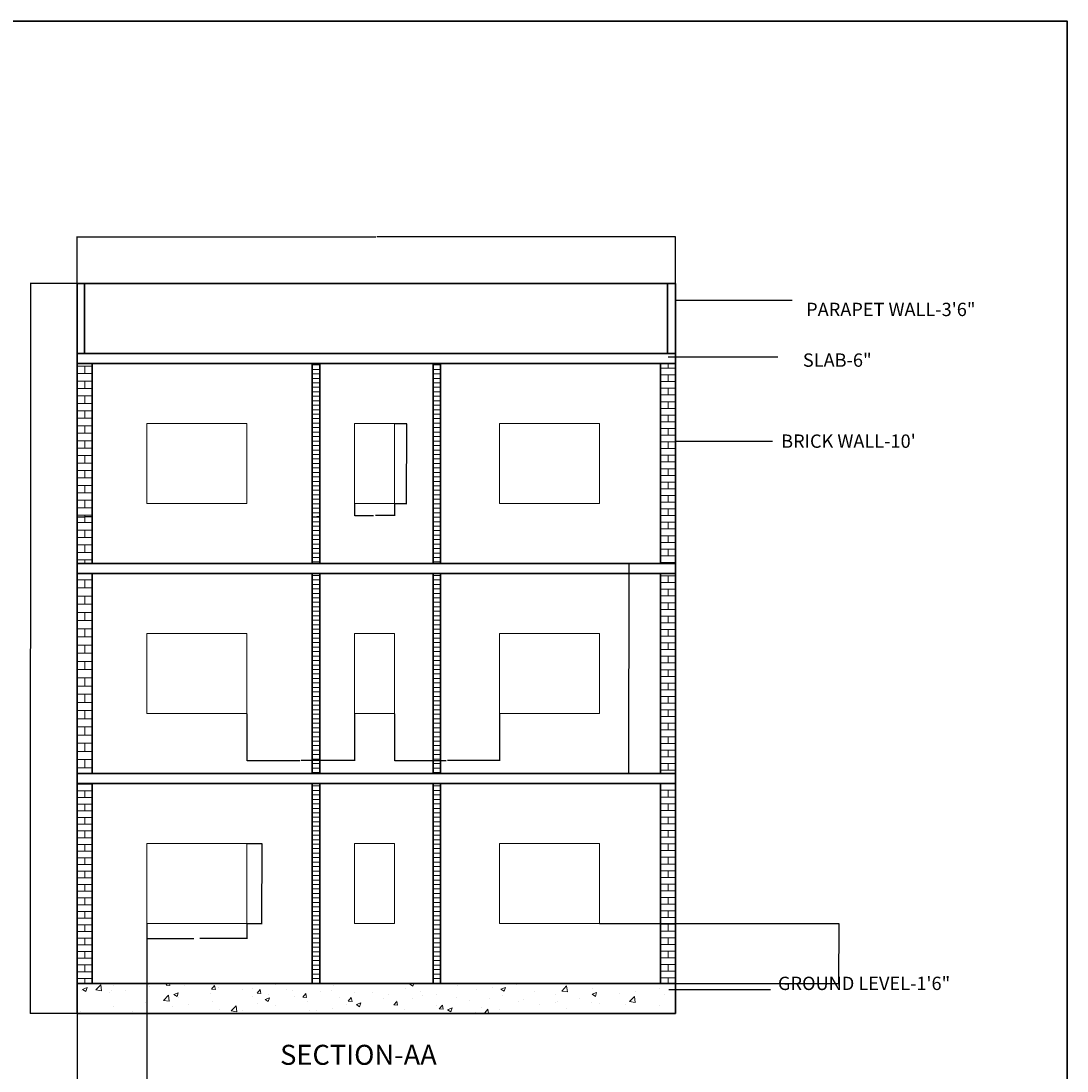
# Model space of a CAD drawing. Units: inches. Extents: x 1832 to 2989, y 1644 to 2902.
# Tile 8 of 8: x 2361 to 2989, y 2272 to 2902. Entities that reach past the tile are written whole.
import ezdxf

# ---------------------------------------------------------------- set-up
doc = ezdxf.new("R2010")
doc.units = ezdxf.units.IN
for name, color, linetype, lineweight in [('A-ANNO-DIMS', 2, 'Continuous', 18), ('A-ANNO-TEXT', 7, 'Continuous', 25), ('A-ANNO-TTLB', 7, 'Continuous', 35), ('A-SECT', 7, 'Continuous', 35), ('A-SECT-GLAZ', 4, 'Continuous', 18), ('A-SECT-PATT', 252, 'Continuous', 13), ('A-WALL-PATT', 252, 'Continuous', 13)]:
    doc.layers.add(name, color=color, linetype=linetype, lineweight=lineweight)
doc.styles.get("Standard").update_dxf_attribs({"font": 'arial.ttf'})
doc.dimstyles.get("Standard").update_dxf_attribs({"dimtxt": 0.18, "dimasz": 0.18, "dimexe": 0.18, "dimexo": 0.0625, "dimgap": 0.09, "dimtad": 0, "dimtih": 1, "dimtoh": 1, "dimdec": 4, "dimzin": 0, "dimdsep": 46, "dimtxsty": 'Standard', "dimcen": 0.09, "dimadec": 0, "dimazin": 0, "dimtfac": 1, "dimtdec": 4, "dimtofl": 0, "dimtmove": 0, "dimatfit": 3, "dimfxl": 1, "dimtolj": 1, "dimtzin": 0, "dimarcsym": 0})

# ---------------------------------------------------------------- blocks, each defined once
blk = doc.blocks.new('WIN-SECT-60IN')
for p, q in [((0, 0), (0, 48)), ((60, 48), (0, 48)), ((60, 0), (60, 48)), ((60, 0), (0, 0))]:
    blk.add_line(p, q)
blk = doc.blocks.new('WIN-SECT-24IN')
for p, q in [((0, 48), (0, 0)), ((24, 48), (0, 48)), ((24, 48), (24, 0)), ((24, 0), (0, 0))]:
    blk.add_line(p, q)
blk = doc.blocks.new('*D67')
at = {"layer": 'A-ANNO-DIMS', "color": 0, "lineweight": -2, "transparency": 16777216}
for p, q in [((2436.72, 2360.25), (2436.72, 2351.13)), ((2496.72, 2360.25), (2496.72, 2351.13)), ((2436.9, 2351.31), (2464.92, 2351.31)), ((2496.54, 2351.31), (2468.51, 2351.31))]:
    blk.add_line(p, q, dxfattribs=at)
at = {"layer": 'A-ANNO-DIMS', "color": 0, "transparency": 16777216}
for points in [[(2436.9, 2351.34), (2436.9, 2351.28), (2436.72, 2351.31)], [(2496.54, 2351.34), (2496.54, 2351.28), (2496.72, 2351.31)]]:
    blk.add_solid(points, dxfattribs=at)
at = {"layer": 'Defpoints', "color": 0, "transparency": 16777216}
for p in [(2436.72, 2360.31), (2496.72, 2360.31), (2496.72, 2351.31)]:
    blk.add_point(p, dxfattribs=at)
at = {"layer": 'A-ANNO-DIMS', "color": 0, "transparency": 16777216, "insert": (2466.72, 2351.31), "char_height": 0.18, "attachment_point": 5}
blk.add_mtext('\\A1;BEDROOM WINDOW 60 TYP.', dxfattribs=at)
blk = doc.blocks.new('*D68')
at = {"layer": 'A-ANNO-DIMS', "color": 0, "lineweight": -2, "transparency": 16777216}
for p, q in [((2496.78, 2408.31), (2505.9, 2408.31)), ((2505.72, 2408.13), (2505.72, 2384.49)), ((2505.72, 2360.49), (2505.72, 2384.13)), ((2496.78, 2360.31), (2505.9, 2360.31))]:
    blk.add_line(p, q, dxfattribs=at)
at = {"layer": 'A-ANNO-DIMS', "color": 0, "transparency": 16777216}
for points in [[(2505.69, 2408.13), (2505.75, 2408.13), (2505.72, 2408.31)], [(2505.69, 2360.49), (2505.75, 2360.49), (2505.72, 2360.31)]]:
    blk.add_solid(points, dxfattribs=at)
at = {"layer": 'Defpoints', "color": 0, "transparency": 16777216}
for p in [(2496.72, 2408.31), (2505.72, 2408.31), (2496.72, 2360.31)]:
    blk.add_point(p, dxfattribs=at)
at = {"layer": 'A-ANNO-DIMS', "color": 0, "transparency": 16777216, "insert": (2505.72, 2384.31), "char_height": 0.18, "attachment_point": 5}
blk.add_mtext('\\A1;48 TYP.', dxfattribs=at)
blk = doc.blocks.new('*D69')
at = {"layer": 'A-ANNO-DIMS', "color": 0, "lineweight": -2, "transparency": 16777216}
for p, q in [((2585.42, 2660.31), (2592.74, 2660.31)), ((2592.56, 2660.13), (2592.56, 2636.5)), ((2592.56, 2612.49), (2592.56, 2636.13)), ((2585.42, 2612.31), (2592.74, 2612.31))]:
    blk.add_line(p, q, dxfattribs=at)
at = {"layer": 'A-ANNO-DIMS', "color": 0, "transparency": 16777216}
for points in [[(2592.53, 2660.13), (2592.59, 2660.13), (2592.56, 2660.31)], [(2592.53, 2612.49), (2592.59, 2612.49), (2592.56, 2612.31)]]:
    blk.add_solid(points, dxfattribs=at)
at = {"layer": 'Defpoints', "color": 0, "transparency": 16777216}
for p in [(2585.36, 2660.31), (2592.56, 2660.31), (2585.36, 2612.31)]:
    blk.add_point(p, dxfattribs=at)
at = {"layer": 'A-ANNO-DIMS', "color": 0, "transparency": 16777216, "insert": (2592.56, 2636.31), "char_height": 0.18, "attachment_point": 5}
blk.add_mtext('\\A1;WC WINDOW 48 TYP.', dxfattribs=at)
blk = doc.blocks.new('*D70')
at = {"layer": 'A-ANNO-DIMS', "color": 0, "lineweight": -2, "transparency": 16777216}
for p, q in [((2561.36, 2612.25), (2561.36, 2604.93)), ((2585.36, 2612.25), (2585.36, 2604.93)), ((2561.54, 2605.11), (2572.83, 2605.11)), ((2585.18, 2605.11), (2573.89, 2605.11))]:
    blk.add_line(p, q, dxfattribs=at)
at = {"layer": 'A-ANNO-DIMS', "color": 0, "transparency": 16777216}
for points in [[(2561.54, 2605.14), (2561.54, 2605.08), (2561.36, 2605.11)], [(2585.18, 2605.14), (2585.18, 2605.08), (2585.36, 2605.11)]]:
    blk.add_solid(points, dxfattribs=at)
at = {"layer": 'Defpoints', "color": 0, "transparency": 16777216}
for p in [(2561.36, 2612.31), (2585.36, 2612.31), (2585.36, 2605.11)]:
    blk.add_point(p, dxfattribs=at)
at = {"layer": 'A-ANNO-DIMS', "color": 0, "transparency": 16777216, "insert": (2573.36, 2605.11), "char_height": 0.18, "attachment_point": 5}
blk.add_mtext('\\A1;24 TYP.', dxfattribs=at)
blk = doc.blocks.new('*D113')
at = {"layer": 'A-ANNO-DIMS', "color": 0, "lineweight": -2, "transparency": 16777216}
for p, q in [((2395.04, 2744.37), (2395.04, 2772.54)), ((2395.22, 2772.36), (2574.25, 2772.36)), ((2753.86, 2772.36), (2574.82, 2772.36)), ((2754.04, 2744.37), (2754.04, 2772.54))]:
    blk.add_line(p, q, dxfattribs=at)
at = {"layer": 'A-ANNO-DIMS', "color": 0, "transparency": 16777216}
for points in [[(2395.22, 2772.39), (2395.22, 2772.33), (2395.04, 2772.36)], [(2753.86, 2772.39), (2753.86, 2772.33), (2754.04, 2772.36)]]:
    blk.add_solid(points, dxfattribs=at)
at = {"layer": 'Defpoints', "color": 0, "transparency": 16777216}
for p in [(2754.04, 2772.36), (2395.04, 2744.31), (2754.04, 2744.31)]:
    blk.add_point(p, dxfattribs=at)
at = {"layer": 'A-ANNO-DIMS', "color": 0, "transparency": 16777216, "insert": (2574.54, 2772.36), "char_height": 0.18, "attachment_point": 5}
blk.add_mtext('\\A1;359', dxfattribs=at)
blk = doc.blocks.new('*D114')
at = {"layer": 'A-ANNO-DIMS', "color": 0, "lineweight": -2, "transparency": 16777216}
for p, q in [((2394.97, 2744.31), (2366.81, 2744.31)), ((2366.99, 2744.13), (2366.99, 2525.49)), ((2366.99, 2306.49), (2366.99, 2525.13)), ((2394.97, 2306.31), (2366.81, 2306.31))]:
    blk.add_line(p, q, dxfattribs=at)
at = {"layer": 'A-ANNO-DIMS', "color": 0, "transparency": 16777216}
for points in [[(2366.96, 2744.13), (2367.02, 2744.13), (2366.99, 2744.31)], [(2366.96, 2306.49), (2367.02, 2306.49), (2366.99, 2306.31)]]:
    blk.add_solid(points, dxfattribs=at)
at = {"layer": 'Defpoints', "color": 0, "transparency": 16777216}
for p in [(2366.99, 2744.31), (2395.04, 2744.31), (2395.04, 2306.31)]:
    blk.add_point(p, dxfattribs=at)
at = {"layer": 'A-ANNO-DIMS', "color": 0, "transparency": 16777216, "insert": (2366.99, 2525.31), "char_height": 0.18, "attachment_point": 5}
blk.add_mtext('\\A1;438', dxfattribs=at)
blk = doc.blocks.new('*D115')
at = {"layer": 'A-ANNO-DIMS', "color": 0, "lineweight": -2, "transparency": 16777216}
for p, q in [((2436.72, 2360.25), (2436.72, 2243.31)), ((2395.04, 2306.25), (2395.04, 2243.31)), ((2395.22, 2243.49), (2415.48, 2243.49)), ((2436.54, 2243.49), (2416.27, 2243.49))]:
    blk.add_line(p, q, dxfattribs=at)
at = {"layer": 'A-ANNO-DIMS', "color": 0, "transparency": 16777216}
for points in [[(2395.22, 2243.52), (2395.22, 2243.46), (2395.04, 2243.49)], [(2436.54, 2243.52), (2436.54, 2243.46), (2436.72, 2243.49)]]:
    blk.add_solid(points, dxfattribs=at)
at = {"layer": 'Defpoints', "color": 0, "transparency": 16777216}
for p in [(2436.72, 2360.31), (2395.04, 2306.31), (2436.72, 2243.49)]:
    blk.add_point(p, dxfattribs=at)
at = {"layer": 'A-ANNO-DIMS', "color": 0, "transparency": 16777216, "insert": (2415.88, 2243.49), "char_height": 0.18, "attachment_point": 5}
blk.add_mtext('\\A1;41.68', dxfattribs=at)
blk = doc.blocks.new('*D116')
at = {"layer": 'A-ANNO-DIMS', "color": 0, "lineweight": -2, "transparency": 16777216}
for p, q in [((2496.72, 2486.25), (2496.72, 2458.08)), ((2561.36, 2486.25), (2561.36, 2458.08)), ((2496.9, 2458.26), (2528.64, 2458.26)), ((2561.18, 2458.26), (2529.43, 2458.26))]:
    blk.add_line(p, q, dxfattribs=at)
at = {"layer": 'A-ANNO-DIMS', "color": 0, "transparency": 16777216}
for points in [[(2496.9, 2458.29), (2496.9, 2458.23), (2496.72, 2458.26)], [(2561.18, 2458.29), (2561.18, 2458.23), (2561.36, 2458.26)]]:
    blk.add_solid(points, dxfattribs=at)
at = {"layer": 'Defpoints', "color": 0, "transparency": 16777216}
for p in [(2496.72, 2486.31), (2561.36, 2486.31), (2496.72, 2458.26)]:
    blk.add_point(p, dxfattribs=at)
at = {"layer": 'A-ANNO-DIMS', "color": 0, "transparency": 16777216, "insert": (2529.04, 2458.26), "char_height": 0.18, "attachment_point": 5}
blk.add_mtext('\\A1;64.64', dxfattribs=at)
blk = doc.blocks.new('*D117')
at = {"layer": 'A-ANNO-DIMS', "color": 0, "lineweight": -2, "transparency": 16777216}
for p, q in [((2585.36, 2486.25), (2585.36, 2458.08)), ((2648.39, 2486.25), (2648.39, 2458.08)), ((2585.54, 2458.26), (2616.48, 2458.26)), ((2648.21, 2458.26), (2617.27, 2458.26))]:
    blk.add_line(p, q, dxfattribs=at)
at = {"layer": 'A-ANNO-DIMS', "color": 0, "transparency": 16777216}
for points in [[(2585.54, 2458.29), (2585.54, 2458.23), (2585.36, 2458.26)], [(2648.21, 2458.29), (2648.21, 2458.23), (2648.39, 2458.26)]]:
    blk.add_solid(points, dxfattribs=at)
at = {"layer": 'Defpoints', "color": 0, "transparency": 16777216}
for p in [(2585.36, 2486.31), (2648.39, 2486.31), (2585.36, 2458.26)]:
    blk.add_point(p, dxfattribs=at)
at = {"layer": 'A-ANNO-DIMS', "color": 0, "transparency": 16777216, "insert": (2616.87, 2458.26), "char_height": 0.18, "attachment_point": 5}
blk.add_mtext('\\A1;63.03', dxfattribs=at)
blk = doc.blocks.new('*D118')
at = {"layer": 'A-ANNO-DIMS', "color": 0, "lineweight": -2, "transparency": 16777216}
for p, q in [((2753.97, 2576.31), (2725.81, 2576.31)), ((2725.99, 2576.13), (2725.99, 2513.49)), ((2725.99, 2450.49), (2725.99, 2513.13)), ((2753.97, 2450.31), (2725.81, 2450.31))]:
    blk.add_line(p, q, dxfattribs=at)
at = {"layer": 'A-ANNO-DIMS', "color": 0, "transparency": 16777216}
for points in [[(2725.96, 2576.13), (2726.02, 2576.13), (2725.99, 2576.31)], [(2725.96, 2450.49), (2726.02, 2450.49), (2725.99, 2450.31)]]:
    blk.add_solid(points, dxfattribs=at)
at = {"layer": 'Defpoints', "color": 0, "transparency": 16777216}
for p in [(2725.99, 2576.31), (2754.04, 2576.31), (2754.04, 2450.31)]:
    blk.add_point(p, dxfattribs=at)
at = {"layer": 'A-ANNO-DIMS', "color": 0, "transparency": 16777216, "insert": (2725.99, 2513.31), "char_height": 0.18, "attachment_point": 5}
blk.add_mtext('\\A1;126', dxfattribs=at)
blk = doc.blocks.new('*D119')
at = {"layer": 'A-ANNO-DIMS', "color": 0, "lineweight": -2, "transparency": 16777216}
for p, q in [((2708.45, 2360.31), (2852.18, 2360.31)), ((2852, 2360.13), (2852, 2342.49)), ((2852, 2324.49), (2852, 2342.13)), ((2754.1, 2324.31), (2852.18, 2324.31))]:
    blk.add_line(p, q, dxfattribs=at)
at = {"layer": 'A-ANNO-DIMS', "color": 0, "transparency": 16777216}
for points in [[(2851.97, 2360.13), (2852.03, 2360.13), (2852, 2360.31)], [(2851.97, 2324.49), (2852.03, 2324.49), (2852, 2324.31)]]:
    blk.add_solid(points, dxfattribs=at)
at = {"layer": 'Defpoints', "color": 0, "transparency": 16777216}
for p in [(2708.39, 2360.31), (2852, 2360.31), (2754.04, 2324.31)]:
    blk.add_point(p, dxfattribs=at)
at = {"layer": 'A-ANNO-DIMS', "color": 0, "transparency": 16777216, "insert": (2852, 2342.31), "char_height": 0.18, "attachment_point": 5}
blk.add_mtext('\\A1;36', dxfattribs=at)
blk = doc.blocks.new('*D120')
at = {"layer": 'A-ANNO-DIMS', "color": 0, "lineweight": -2, "transparency": 16777216}
for p, q in [((2395.04, 2576.37), (2395.04, 2604.54)), ((2395.22, 2604.36), (2399.39, 2604.36)), ((2403.86, 2604.36), (2399.68, 2604.36)), ((2404.04, 2576.37), (2404.04, 2604.54))]:
    blk.add_line(p, q, dxfattribs=at)
at = {"layer": 'A-ANNO-DIMS', "color": 0, "transparency": 16777216}
for points in [[(2395.22, 2604.39), (2395.22, 2604.33), (2395.04, 2604.36)], [(2403.86, 2604.39), (2403.86, 2604.33), (2404.04, 2604.36)]]:
    blk.add_solid(points, dxfattribs=at)
at = {"layer": 'Defpoints', "color": 0, "transparency": 16777216}
for p in [(2404.04, 2604.36), (2395.04, 2576.31), (2404.04, 2576.31)]:
    blk.add_point(p, dxfattribs=at)
at = {"layer": 'A-ANNO-DIMS', "color": 0, "transparency": 16777216, "insert": (2399.54, 2604.36), "char_height": 0.18, "attachment_point": 5}
blk.add_mtext('\\A1;9', dxfattribs=at)
blk = doc.blocks.new('*D121')
at = {"layer": 'A-ANNO-DIMS', "color": 0, "lineweight": -2, "transparency": 16777216}
for p, q in [((2536.04, 2576.37), (2536.04, 2604.54)), ((2536.22, 2604.36), (2538.03, 2604.36)), ((2540.36, 2604.36), (2538.54, 2604.36)), ((2540.54, 2576.37), (2540.54, 2604.54))]:
    blk.add_line(p, q, dxfattribs=at)
at = {"layer": 'A-ANNO-DIMS', "color": 0, "transparency": 16777216}
for points in [[(2536.22, 2604.39), (2536.22, 2604.33), (2536.04, 2604.36)], [(2540.36, 2604.39), (2540.36, 2604.33), (2540.54, 2604.36)]]:
    blk.add_solid(points, dxfattribs=at)
at = {"layer": 'Defpoints', "color": 0, "transparency": 16777216}
for p in [(2540.54, 2604.36), (2536.04, 2576.31), (2540.54, 2576.31)]:
    blk.add_point(p, dxfattribs=at)
at = {"layer": 'A-ANNO-DIMS', "color": 0, "transparency": 16777216, "insert": (2538.29, 2604.36), "char_height": 0.18, "attachment_point": 5}
blk.add_mtext('\\A1;4.5', dxfattribs=at)

msp = doc.modelspace()

# ---------------------------------------------------------------- hatches: boundary and pattern name
at = {"layer": 'A-SECT-PATT'}
h = msp.add_hatch(dxfattribs=at)
h.set_pattern_fill('AR-CONC', color=256, scale=0.15, style=0)
h.paths.add_polyline_path([(2395.0354, 2306.3121), (2754.0354, 2306.3121), (2754.0354, 2324.3121), (2395.0354, 2324.3121)])
at = {"layer": 'A-WALL-PATT'}
h = msp.add_hatch(dxfattribs=at)
h.set_pattern_fill('AR-BRSTD', color=256, scale=0.0659706, style=0)
h.paths.add_polyline_path([(2395.0354, 2576.3121), (2404.0354, 2576.3121), (2404.0354, 2696.3121), (2395.0354, 2696.3121)])
h = msp.add_hatch(dxfattribs=at)
h.set_pattern_fill('ANSI31', color=256, scale=0.846457, angle=315, style=0)
h.paths.add_polyline_path([(2536.0354, 2576.3121), (2540.5354, 2576.3121), (2540.5354, 2696.3121), (2536.0354, 2696.3121)])
h = msp.add_hatch(dxfattribs=at)
h.set_pattern_fill('ANSI31', color=256, scale=0.846457, angle=315, style=0)
h.paths.add_polyline_path([(2608.5354, 2576.3121), (2613.0354, 2576.3121), (2613.0354, 2696.3121), (2608.5354, 2696.3121)])
h = msp.add_hatch(dxfattribs=at)
h.set_pattern_fill('AR-BRSTD', color=256, scale=0.0593473, style=0)
h.paths.add_polyline_path([(2745.0354, 2576.3121), (2754.0354, 2576.3121), (2754.0354, 2696.3121), (2745.0354, 2696.3121)])
h = msp.add_hatch(dxfattribs=at)
h.set_pattern_fill('AR-BRSTD', color=256, scale=0.0724462, style=0)
h.paths.add_polyline_path([(2395.0354, 2450.3121), (2404.0354, 2450.3121), (2404.0354, 2570.3121), (2395.0354, 2570.3121)])
h = msp.add_hatch(dxfattribs=at)
h.set_pattern_fill('ANSI31', color=256, scale=0.846457, angle=315, style=0)
h.paths.add_polyline_path([(2536.0354, 2450.3121), (2540.5354, 2450.3121), (2540.5354, 2570.3121), (2536.0354, 2570.3121)])
h = msp.add_hatch(dxfattribs=at)
h.set_pattern_fill('ANSI31', color=256, scale=0.846457, angle=315, style=0)
h.paths.add_polyline_path([(2608.5354, 2450.3121), (2613.0354, 2450.3121), (2613.0354, 2570.3121), (2608.5354, 2570.3121)])
h = msp.add_hatch(dxfattribs=at)
h.set_pattern_fill('AR-BRSTD', color=256, scale=0.0593473, style=0)
h.paths.add_polyline_path([(2745.0354, 2450.3121), (2754.0354, 2450.3121), (2754.0354, 2570.3121), (2745.0354, 2570.3121)])
h = msp.add_hatch(dxfattribs=at)
h.set_pattern_fill('AR-BRSTD', color=256, scale=0.0593404, style=0)
h.paths.add_polyline_path([(2395.0354, 2324.3121), (2404.0354, 2324.3121), (2404.0354, 2444.3121), (2395.0354, 2444.3121)])
h = msp.add_hatch(dxfattribs=at)
h.set_pattern_fill('ANSI31', color=256, scale=0.846457, angle=315, style=0)
h.paths.add_polyline_path([(2536.0354, 2324.3121), (2540.5354, 2324.3121), (2540.5354, 2444.3121), (2536.0354, 2444.3121)])
h = msp.add_hatch(dxfattribs=at)
h.set_pattern_fill('ANSI31', color=256, scale=0.846457, angle=315, style=0)
h.paths.add_polyline_path([(2608.5354, 2324.3121), (2613.0354, 2324.3121), (2613.0354, 2444.3121), (2608.5354, 2444.3121)])
h = msp.add_hatch(dxfattribs=at)
h.set_pattern_fill('AR-BRSTD', color=256, scale=0.0593473, style=0)
h.paths.add_polyline_path([(2745.0354, 2324.3121), (2754.0354, 2324.3121), (2754.0354, 2444.3121), (2745.0354, 2444.3121)])

# ---------------------------------------------------------------- linework, layer by layer
at = {"layer": 'A-ANNO-TEXT'}
for p, q in [((2754.0354, 2734.3413), (2823.9485, 2734.3413)), ((2749.5985, 2700.3449), (2815.3166, 2700.3449)), ((2812.1753, 2649.5049), (2754.0354, 2649.5049)), ((2749.986, 2320.8492), (2811.0375, 2320.8492))]:
    msp.add_line(p, q, dxfattribs=at)
at = {"layer": 'A-ANNO-TTLB'}
msp.add_lwpolyline([(1831.6677, 2901.9044), (2988.9144, 2901.9044), (2988.9144, 1643.5851), (1831.6677, 1643.5851)], close=True, dxfattribs=at)
at = {"layer": 'A-SECT'}
for p, q in [((2395.0354, 2744.3121), (2395.0354, 2558.3121)), ((2754.0354, 2744.3121), (2395.0354, 2744.3121)), ((2399.3636, 2702.3121), (2399.3636, 2744.3121)), ((2749.1205, 2702.3121), (2749.1205, 2744.3121)), ((2754.0354, 2744.3121), (2754.0354, 2558.3121)), ((2754.0354, 2702.3121), (2395.0354, 2702.3121)), ((2754.0354, 2696.3121), (2395.0354, 2696.3121)), ((2404.0354, 2696.3121), (2404.0354, 2576.3121)), ((2536.0354, 2696.3121), (2536.0354, 2576.3121)), ((2540.5354, 2696.3121), (2540.5354, 2576.3121)), ((2608.5354, 2696.3121), (2608.5354, 2576.3121)), ((2613.0354, 2696.3121), (2613.0354, 2576.3121)), ((2745.0354, 2696.3121), (2745.0354, 2576.3121)), ((2395.0354, 2618.3121), (2395.0354, 2432.3121)), ((2754.0354, 2618.3121), (2754.0354, 2432.3121)), ((2754.0354, 2576.3121), (2395.0354, 2576.3121)), ((2754.0354, 2570.3121), (2395.0354, 2570.3121)), ((2404.0354, 2570.3121), (2404.0354, 2450.3121)), ((2536.0354, 2570.3121), (2536.0354, 2450.3121)), ((2540.5354, 2570.3121), (2540.5354, 2450.3121)), ((2608.5354, 2570.3121), (2608.5354, 2450.3121)), ((2613.0354, 2570.3121), (2613.0354, 2450.3121)), ((2745.0354, 2570.3121), (2745.0354, 2450.3121)), ((2395.0354, 2492.3121), (2395.0354, 2306.3121)), ((2754.0354, 2492.3121), (2754.0354, 2306.3121)), ((2754.0354, 2450.3121), (2395.0354, 2450.3121)), ((2754.0354, 2444.3121), (2395.0354, 2444.3121)), ((2404.0354, 2444.3121), (2404.0354, 2324.3121)), ((2536.0354, 2444.3121), (2536.0354, 2324.3121)), ((2540.5354, 2444.3121), (2540.5354, 2324.3121)), ((2608.5354, 2444.3121), (2608.5354, 2324.3121)), ((2613.0354, 2444.3121), (2613.0354, 2324.3121)), ((2745.0354, 2444.3121), (2745.0354, 2324.3121)), ((2754.0354, 2324.3121), (2395.0354, 2324.3121)), ((2754.0354, 2306.3121), (2395.0354, 2306.3121))]:
    msp.add_line(p, q, dxfattribs=at)

# ---------------------------------------------------------------- block references
at = {"layer": 'A-SECT-GLAZ'}
for name, p in [('WIN-SECT-60IN', (2436.7169, 2612.3121)), ('WIN-SECT-24IN', (2561.3579, 2612.3121)), ('WIN-SECT-60IN', (2648.3901, 2612.3121)), ('WIN-SECT-60IN', (2436.7169, 2486.3121)), ('WIN-SECT-24IN', (2561.3579, 2486.3121)), ('WIN-SECT-60IN', (2648.3901, 2486.3121)), ('WIN-SECT-60IN', (2436.7169, 2360.3121)), ('WIN-SECT-24IN', (2561.3579, 2360.3121)), ('WIN-SECT-60IN', (2648.3901, 2360.3121))]:
    msp.add_blockref(name, p, dxfattribs=at)

# ---------------------------------------------------------------- texts
at = {"layer": 'A-ANNO-TEXT', "attachment_point": 1}
for s, width, insert, char_height in [('PARAPET WALL-3\'6"', 194.123767, (2832.3939, 2732.853), 8), ('SLAB-6"', 70.888027, (2830.425, 2702.4414), 8), ("BRICK WALL-10'", 95.192237, (2817.3885, 2653.8086), 8), ('GROUND LEVEL-1\'6"', 130.994238, (2815.4797, 2328.485), 8), ('SECTION-AA', 223.733993, (2516.7492, 2287.6181), 12)]:
    msp.add_mtext_dynamic_manual_height_columns(s, width=width, gutter_width=12.5, heights=[0], dxfattribs=dict(at, insert=insert, char_height=char_height))

# ---------------------------------------------------------------- dimensions: what is measured, and where the dimension line sits
at = {"layer": 'A-ANNO-DIMS'}
for base, p1, p2, override, picture, middle in [((2754.0354, 2772.3621), (2395.0354, 2744.3121), (2754.0354, 2744.3121), {"dimdec": 0, "dimlfac": 1, "dimrnd": 0, "dimzin": 0, "dimdsep": 46, "dimlunit": 2}, '*D113', (2574.5354, 2772.3621)), ((2404.0354, 2604.3621), (2395.0354, 2576.3121), (2404.0354, 2576.3121), {"dimdec": 0, "dimlfac": 1, "dimrnd": 0, "dimzin": 0, "dimdsep": 46, "dimlunit": 2}, '*D120', (2399.5354, 2604.3621)), ((2540.5354, 2604.3621), (2536.0354, 2576.3121), (2540.5354, 2576.3121), {"dimdec": 1, "dimlfac": 1, "dimrnd": 0, "dimzin": 0, "dimdsep": 46, "dimlunit": 2}, '*D121', (2538.2854, 2604.3621)), ((2436.7169, 2243.4866), (2395.0354, 2306.3121), (2436.7169, 2360.3121), {"dimdec": 2, "dimlfac": 1, "dimrnd": 0, "dimzin": 0, "dimdsep": 46, "dimlunit": 2}, '*D115', (2415.8762, 2243.4866))]:
    dim = msp.add_linear_dim(base=base, p1=p1, p2=p2, dimstyle='Standard', override=override, dxfattribs=at)
    dim.commit()
    dim.dimension.update_dxf_attribs({"geometry": picture, "text_midpoint": middle})
for base, p1, p2, angle, override, picture, middle in [((2366.9854, 2744.3121), (2395.0354, 2306.3121), (2395.0354, 2744.3121), 90, {"dimdec": 0, "dimlfac": 1, "dimrnd": 0, "dimzin": 0, "dimdsep": 46, "dimlunit": 2}, '*D114', (2366.9854, 2525.3121)), ((2725.9854, 2576.3121), (2754.0354, 2450.3121), (2754.0354, 2576.3121), 90, {"dimdec": 0, "dimlfac": 1, "dimrnd": 0, "dimzin": 0, "dimdsep": 46, "dimlunit": 2}, '*D118', (2725.9854, 2513.3121)), ((2496.7169, 2458.2621), (2561.3579, 2486.3121), (2496.7169, 2486.3121), 180, {"dimdec": 2, "dimlfac": 1, "dimrnd": 0, "dimzin": 0, "dimdsep": 46, "dimlunit": 2}, '*D116', (2529.0374, 2458.2621)), ((2585.3579, 2458.2621), (2648.3901, 2486.3121), (2585.3579, 2486.3121), 180, {"dimdec": 2, "dimlfac": 1, "dimrnd": 0, "dimzin": 0, "dimdsep": 46, "dimlunit": 2}, '*D117', (2616.874, 2458.2621)), ((2851.9985, 2360.3121), (2754.0354, 2324.3121), (2708.3901, 2360.3121), 90, {"dimdec": 0, "dimlfac": 1, "dimrnd": 0, "dimzin": 0, "dimdsep": 46, "dimlunit": 2}, '*D119', (2851.9985, 2342.3121))]:
    dim = msp.add_linear_dim(base=base, p1=p1, p2=p2, angle=angle, dimstyle='Standard', override=override, dxfattribs=at)
    dim.commit()
    dim.dimension.update_dxf_attribs({"geometry": picture, "text_midpoint": middle})
for base, p1, p2, text, picture, middle in [((2592.5579, 2660.3121), (2585.3579, 2612.3121), (2585.3579, 2660.3121), 'WC WINDOW <> TYP.', '*D69', (2592.5579, 2636.3121)), ((2505.7169, 2408.3121), (2496.7169, 2360.3121), (2496.7169, 2408.3121), '<> TYP.', '*D68', (2505.7169, 2384.3121))]:
    dim = msp.add_linear_dim(base=base, p1=p1, p2=p2, angle=90, text=text, dimstyle='Standard', override={"dimdec": 0, "dimlfac": 1, "dimrnd": 0, "dimzin": 0, "dimdsep": 46, "dimlunit": 2}, dxfattribs=at)
    dim.commit()
    dim.dimension.update_dxf_attribs({"geometry": picture, "text_midpoint": middle})
for base, p1, p2, text, picture, middle in [((2585.3579, 2605.1121), (2561.3579, 2612.3121), (2585.3579, 2612.3121), '<> TYP.', '*D70', (2573.3579, 2605.1121)), ((2496.7169, 2351.3121), (2436.7169, 2360.3121), (2496.7169, 2360.3121), 'BEDROOM WINDOW <> TYP.', '*D67', (2466.7169, 2351.3121))]:
    dim = msp.add_linear_dim(base=base, p1=p1, p2=p2, text=text, dimstyle='Standard', override={"dimdec": 0, "dimlfac": 1, "dimrnd": 0, "dimzin": 0, "dimdsep": 46, "dimlunit": 2}, dxfattribs=at)
    dim.commit()
    dim.dimension.update_dxf_attribs({"geometry": picture, "text_midpoint": middle})

doc.saveas('drawing.dxf')
